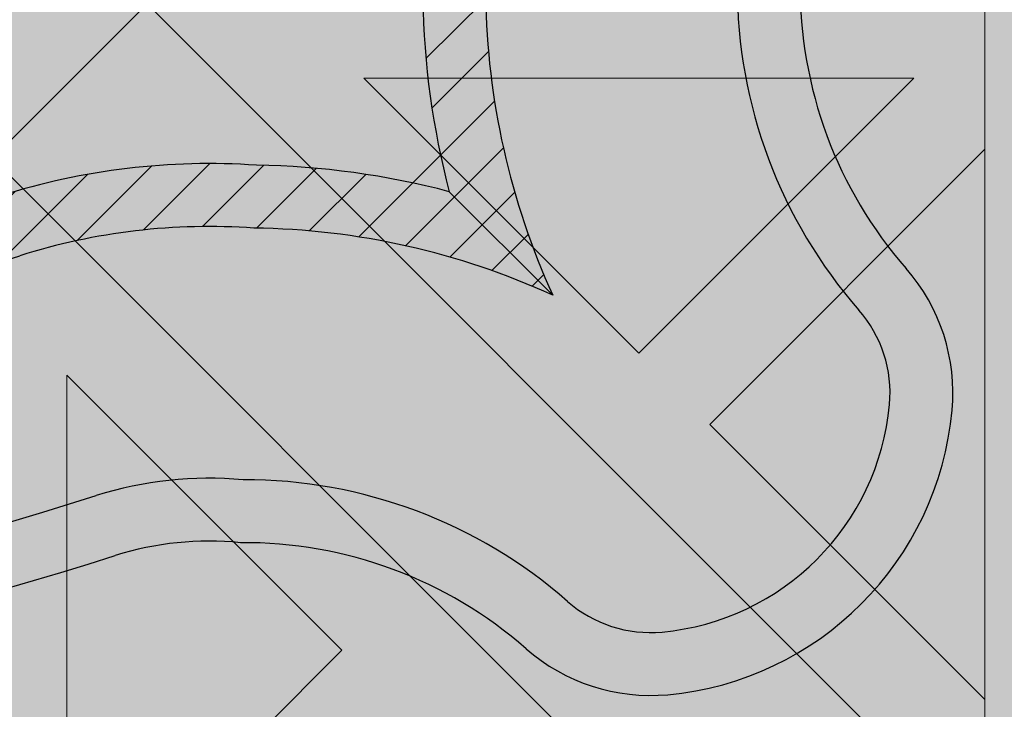
# Model space of a CAD drawing. Units: inches. Extents: x 844 to 2234, y 346 to 1084.
# Tile 54 of 93: x 1871.357 to 1873.853, y 692.527 to 694.275. Entities that reach past the tile are written whole.
import ezdxf

# ---------------------------------------------------------------- set-up
doc = ezdxf.new("R2010")
doc.units = ezdxf.units.IN
doc.header["$MEASUREMENT"] = 0
doc.layers.add('furniture', color=8, linetype='Continuous', lineweight=18)
doc.layers.add('RA-AP-01$0$INT', color=35, linetype='Continuous', lineweight=5)
doc.layers.add('RA-AP-01$0$FURN', color=3, linetype='Continuous')
doc.layers.add('RA-AP-01$0$WOOD', color=64, linetype='Continuous')

# ---------------------------------------------------------------- blocks, each defined once
blk = doc.blocks.new('A$C18D01794')
at = {"layer": 'RA-AP-01$0$INT'}
blk.add_hatch(color=256, dxfattribs=at).paths.add_polyline_path([(4.505206456958071, -6.306712009588038), (5.305206456958072, -6.306712009588038), (5.305206456958072, -7.106712009588038), (5.255206456951893, -7.10671200958804), (5.25520645694868, -6.356712009605972), (4.555206456959269, -6.356712009587461), (4.555206456956052, -7.106712009588038), (4.505206456958073, -7.106712009588038)])
h = blk.add_hatch(color=256, dxfattribs=at)
h.paths.add_polyline_path([(4.585917135068449, -6.356712009588271), (4.555206456959269, -6.35671200958746), (4.555206456959137, -6.387422687716308), (4.874495778835233, -6.706712009592356), (4.90520645695423, -6.676001331474049)])
h.paths.add_polyline_path([(5.255206456948813, -6.387422687716306), (5.255206456948682, -6.356712009605972), (5.224495778822613, -6.356712009605161), (4.905206456953498, -6.676001331474273), (4.935917135072151, -6.706712009592924)])
h.paths.add_polyline_path([(4.935917135072559, -6.706712009592068), (4.905206456953564, -6.737422687710376), (5.255206456951813, -7.087422687708613), (5.255206456951549, -7.026001331471008)])
h.paths.add_polyline_path([(4.555206456956399, -7.026001331471013), (4.555206456956134, -7.087422687708616), (4.905206456953821, -6.737422687710943), (4.874495778835166, -6.70671200959229)])
h = blk.add_hatch(color=256, dxfattribs=at)
h.paths.add_polyline_path([(4.585917135068448, -6.356712009588273), (4.614201406330596, -6.356712009589021), (4.668846067270487, -6.411356670531338), (4.723490728212344, -6.356712009591912), (4.771774999457151, -6.35671200959319), (4.826419660396886, -6.411356670535356), (4.862780050090322, -6.374996280843536), (4.844495778842715, -6.356712009595112), (4.862780050090411, -6.356712009595595), (4.905206456960182, -6.399138416468211), (4.947632863832445, -6.356712009597838), (4.965917135079675, -6.356712009598322), (4.947632863831759, -6.374996280845421), (4.983993253523576, -6.411356670538857), (5.038637914464627, -6.356712009600247), (5.08692218571208, -6.356712009601523), (5.141566846649976, -6.411356670541852), (5.196211507589851, -6.356712009604411), (5.224495778822615, -6.356712009605161), (4.905206456953975, -6.676001331473793)])
h.paths.add_polyline_path([(4.895206456956031, -6.637717060225675), (4.895206456958921, -6.528427738347902), (4.840561796018589, -6.583072399285802)], flags=16)
h.paths.add_polyline_path([(4.915206456955638, -6.637717060226121), (4.969851117895509, -6.583072399288678), (4.915206456957609, -6.528427738348344)], flags=16)
h.paths.add_polyline_path([(4.826419660395175, -6.568930263661755), (4.881064321335613, -6.514285602723745), (4.771774999456703, -6.514285602720857)], flags=16)
h.paths.add_polyline_path([(4.983993253519558, -6.568930263665262), (5.038637914460456, -6.514285602726792), (4.929348592581548, -6.514285602724816)], flags=16)
h.paths.add_polyline_path([(4.881064321336025, -6.494285602723742), (4.826419660397532, -6.439640941782821), (4.771774999457062, -6.494285602720859)], flags=16)
h.paths.add_polyline_path([(4.929348592582019, -6.494285602724817), (5.038637914460982, -6.494285602726792), (4.983993253522945, -6.439640941786327)], flags=16)
h.paths.add_polyline_path([(4.895206456960191, -6.480143467100443), (4.895206456962115, -6.407422687715913), (4.876922185715016, -6.389138416467584), (4.840561796021581, -6.425498806159401)], flags=16)
h.paths.add_polyline_path([(4.915206456958487, -6.480143467100889), (4.969851117899527, -6.425498806162279), (4.933490728206909, -6.389138416468043), (4.9152064569598, -6.40742268771434)], flags=16)
h.paths.add_polyline_path([(4.757632863832376, -6.480143467096812), (4.812277524772842, -6.425498806158772), (4.757632863834348, -6.370854145217844)], flags=16)
h.paths.add_polyline_path([(4.737632863832376, -6.480143467096286), (4.737632863834348, -6.370854145217375), (4.682988202893906, -6.425498806155385)], flags=16)
h.paths.add_polyline_path([(5.05278005008503, -6.480143467103376), (5.052780050087917, -6.370854145224413), (4.998135389146995, -6.425498806162908)], flags=16)
h.paths.add_polyline_path([(5.072780050085024, -6.480143467103744), (5.127424711025931, -6.42549880616527), (5.072780050087916, -6.370854145224832)], flags=16)
h.paths.add_polyline_path([(4.935917135072783, -6.706712009592292), (5.255206456948811, -6.387422687716309), (5.255206456948932, -6.415706958964177), (5.200561796010279, -6.470351619902839), (5.255206456949403, -6.524996280841948), (5.25520645694961, -6.5732805520894), (5.200561796009787, -6.627925213029239), (5.236922185702417, -6.664285602721864), (5.255206456949919, -6.646001331474357), (5.255206456949998, -6.664285602721898), (5.212780050078687, -6.706712009592262), (5.25520645695036, -6.749138416463932), (5.255206456950438, -6.767422687711313), (5.236922185702424, -6.749138416463297), (5.200561796009796, -6.785498806155928), (5.255206456950753, -6.840143467096874), (5.25520645695096, -6.888427738341682), (5.200561796010322, -6.943072399282328), (5.255206456951428, -6.997717060223427), (5.255206456951547, -7.026001331471006)])
h.paths.add_polyline_path([(5.042988202883395, -6.785498806155427), (5.097632863823085, -6.840143467095101), (5.097632863822622, -6.730854145216193)], flags=16)
h.paths.add_polyline_path([(5.028846067259663, -6.771356670531693), (5.083490728198774, -6.716712009592573), (4.974201406321001, -6.716712009593042)], flags=16)
h.paths.add_polyline_path([(5.117632863823087, -6.840143467095186), (5.172277524762331, -6.785498806155926), (5.11763286382262, -6.730854145216225)], flags=16)
h.paths.add_polyline_path([(5.08349072819877, -6.696712009593886), (5.028846067259652, -6.642067348654775), (4.974201406320998, -6.696712009593438)], flags=16)
h.paths.add_polyline_path([(5.131774999446817, -6.854285602718917), (5.186419660386065, -6.799640941779662), (5.241064321325782, -6.854285602719365)], flags=17)
h.paths.add_polyline_path([(5.131774999446228, -6.716712009592374), (5.186419660386065, -6.771356670532194), (5.222780050079488, -6.734996280838764), (5.204495778832781, -6.716712009592063)], flags=16)
h.paths.add_polyline_path([(5.097632863822613, -6.682569873970264), (5.097632863823061, -6.573280552091354), (5.042988202883383, -6.627925213031044)], flags=16)
h.paths.add_polyline_path([(5.131774999446899, -6.874285602718915), (5.241064321325809, -6.874285602719364), (5.186419660386591, -6.928930263658598)], flags=17)
h.paths.add_polyline_path([(5.131774999446226, -6.696712009594078), (5.204495778830767, -6.696712009594374), (5.22278005007868, -6.67842773834687), (5.186419660386049, -6.642067348654249)], flags=16)
h.paths.add_polyline_path([(5.11763286382262, -6.682569873970225), (5.17227752476232, -6.627925213030515), (5.117632863823064, -6.573280552091267)], flags=16)
h.paths.add_polyline_path([(5.186419660386069, -6.613783077405491), (5.241064321325754, -6.559138416465795), (5.131774999446791, -6.559138416466263)], flags=16)
h.paths.add_polyline_path([(5.131774999446872, -6.539138416466263), (5.24106432132578, -6.539138416465794), (5.186419660386554, -6.484493755526573)], flags=16)
h.paths.add_polyline_path([(5.255206456951811, -7.08742268770861), (5.255206456951895, -7.106712009588038), (4.555206456956052, -7.106712009588038), (4.555206456956136, -7.087422687708617), (4.905206456953973, -6.737422687710788)])
h.paths.add_polyline_path([(4.983993253513404, -6.8444937555241), (4.92934859257295, -6.899138416462108), (5.03863791445186, -6.899138416465014)], flags=16)
h.paths.add_polyline_path([(4.969851117889988, -6.83035161990006), (4.915206456952556, -6.775706958960171), (4.915206456949648, -6.884996280837944)], flags=16)
h.paths.add_polyline_path([(4.929348592572535, -6.919138416462105), (4.983993253511019, -6.973783077403037), (5.038637914451496, -6.919138416465012)], flags=16)
h.paths.add_polyline_path([(5.052780050074912, -6.93328055208906), (4.998135389134438, -6.987925213027088), (5.052780050072919, -7.042569873968025)], flags=16)
h.paths.add_polyline_path([(5.07278005007491, -6.933280552089588), (5.072780050072918, -7.042569873968497), (5.127424711013374, -6.987925213030498)], flags=16)
h.paths.add_polyline_path([(4.89520645695295, -6.775706958959721), (4.840561796013067, -6.830351619897157), (4.895206456950961, -6.884996280837494)], flags=16)
h.paths.add_polyline_path([(4.915206456948365, -6.933280552085403), (4.915206456946434, -7.006001331471951), (4.933490728192729, -7.024285602719066), (4.969851117886972, -6.987925213026453)], flags=16)
h.paths.add_polyline_path([(4.881064321327021, -6.899138416461022), (4.82641966038902, -6.84449375552057), (4.771774999448108, -6.899138416459029)], flags=16)
h.paths.add_polyline_path([(4.895206456950073, -6.933280552084951), (4.840561796009022, -6.987925213023558), (4.876922185700835, -7.024285602716997), (4.895206456948749, -7.006001331469487)], flags=16)
h.paths.add_polyline_path([(4.983993253510392, -7.0020673486505), (4.947632863816944, -7.038427738342319), (4.965917135064043, -7.05671200959023), (5.038637914448995, -7.056712009591555)], flags=16)
h.paths.add_polyline_path([(4.881064321326543, -6.91913841646102), (4.771774999447578, -6.919138416459031), (4.826419660385607, -6.973783077399508)], flags=16)
h.paths.add_polyline_path([(4.905206456946447, -7.014285602717636), (4.862780050074785, -7.056712009588352), (4.947632863816685, -7.056712009589775)], flags=16)
h.paths.add_polyline_path([(5.14156684663679, -7.002067348654549), (5.086922185696452, -7.056712009592438), (5.196211507574223, -7.056712009594425)], flags=16)
h.paths.add_polyline_path([(4.8264196603837, -7.002067348646972), (4.771774999442643, -7.056712009585575), (4.8444957788276, -7.056712009587508), (4.862780050075511, -7.038427738340416)], flags=16)
h.paths.add_polyline_path([(4.812277524760289, -6.98792521302292), (4.757632863822258, -6.933280552082447), (4.757632863819352, -7.042569873961408)], flags=16)
h.paths.add_polyline_path([(4.73763286382226, -6.933280552082079), (4.682988202881349, -6.987925213020536), (4.737632863819352, -7.04256987396099)], flags=16)
h.paths.add_polyline_path([(4.723490728195188, -7.056712009584289), (4.668846067257299, -7.002067348643949), (4.614201406317417, -7.056712009581383)], flags=16)
h.paths.add_polyline_path([(4.597632863829262, -6.706712009592262), (4.555206456957951, -6.664285602721896), (4.555206456958029, -6.646001331474357), (4.573490728205535, -6.664285602721864), (4.609851117898167, -6.627925213029238), (4.555206456958338, -6.573280552089402), (4.555206456958546, -6.524996280841952), (4.60985111789767, -6.470351619902839), (4.555206456959015, -6.415706958964177), (4.555206456959138, -6.387422687716309), (4.874495778835167, -6.70671200959229), (4.5552064569564, -7.026001331471015), (4.555206456956523, -6.997717060223433), (4.609851117897629, -6.94307239928233), (4.555206456956988, -6.888427738341681), (4.555206456957198, -6.840143467096881), (4.609851117898153, -6.78549880615593), (4.573490728205528, -6.749138416463297), (4.555206456957507, -6.76742268771132), (4.555206456957585, -6.749138416463933)])
h.paths.add_polyline_path([(4.712780050085332, -6.730854145216195), (4.712780050084863, -6.840143467095105), (4.767424711024555, -6.785498806155427)], flags=16)
h.paths.add_polyline_path([(4.726922185709173, -6.716712009592573), (4.781566846648288, -6.771356670531693), (4.836211507586949, -6.716712009593043)], flags=16)
h.paths.add_polyline_path([(4.692780050085327, -6.730854145216225), (4.638135389145619, -6.785498806155928), (4.692780050084865, -6.840143467095185)], flags=16)
h.paths.add_polyline_path([(4.726922185709182, -6.696712009593886), (4.836211507586949, -6.696712009593436), (4.7815668466483, -6.642067348654773)], flags=16)
h.paths.add_polyline_path([(4.678637914461726, -6.71671200959237), (4.605917135075169, -6.716712009592063), (4.587632863828464, -6.734996280838766), (4.623993253521887, -6.771356670532195)], flags=16)
h.paths.add_polyline_path([(4.712780050085336, -6.68256987397026), (4.767424711024568, -6.627925213031042), (4.71278005008489, -6.573280552091352)], flags=16)
h.paths.add_polyline_path([(4.678637914461726, -6.696712009594076), (4.623993253521899, -6.642067348654247), (4.587632863829271, -6.67842773834687), (4.605917135077185, -6.696712009594376)], flags=16)
h.paths.add_polyline_path([(4.692780050085336, -6.682569873970228), (4.692780050084889, -6.573280552091267), (4.638135389145632, -6.627925213030515)], flags=16)
h.paths.add_polyline_path([(4.623993253521885, -6.799640941779662), (4.678637914461131, -6.854285602718915), (4.56934859258217, -6.854285602719365)], flags=17)
h.paths.add_polyline_path([(4.623993253521901, -6.613783077405509), (4.678637914461158, -6.559138416466263), (4.569348592582195, -6.559138416465795)], flags=16)
h.paths.add_polyline_path([(4.678637914461051, -6.874285602718915), (4.623993253521361, -6.928930263658598), (4.569348592582143, -6.874285602719364)], flags=17)
h.paths.add_polyline_path([(4.678637914461076, -6.539138416466263), (4.623993253521399, -6.484493755526573), (4.569348592582167, -6.539138416465796)], flags=16)
h = blk.add_hatch(color=256, dxfattribs=at)
h.paths.add_polyline_path([(4.969851117891331, -6.583072399286455), (4.915206456952669, -6.63771706022511), (4.915206456952222, -6.528427738347337)])
h.paths.add_polyline_path([(4.895206456953064, -6.637717060225108), (4.840561796014413, -6.583072399286448), (4.895206456953533, -6.528427738347335)])
h.paths.add_polyline_path([(4.826419660390684, -6.568930263662714), (4.771774999451003, -6.514285602723024), (4.881064321329913, -6.514285602723489)])
h.paths.add_polyline_path([(4.881064321329884, -6.494285602723492), (4.771774999450921, -6.494285602723024), (4.82641966039018, -6.439640941783778)])
h.paths.add_polyline_path([(4.895206456953734, -6.48014346709988), (4.840561796013912, -6.425498806160046), (4.876922185707337, -6.389138416466622), (4.895206456954043, -6.40742268771333)])
h.paths.add_polyline_path([(4.862780050082808, -6.374996280843689), (4.826419660390178, -6.411356670536314), (4.771774999450351, -6.356712009596481), (4.844495778835303, -6.356712009596181)])
h.paths.add_polyline_path([(4.812277524766446, -6.425498806160041), (4.757632863827191, -6.480143467099289), (4.757632863826741, -6.370854145220329)])
h.paths.add_polyline_path([(4.737632863827191, -6.480143467099214), (4.682988202887508, -6.425498806159518), (4.737632863826743, -6.370854145220299)])
h.paths.add_polyline_path([(4.668846067263777, -6.41135667053579), (4.614201406325123, -6.356712009597128), (4.723490728202894, -6.356712009596675)])
h.paths.add_polyline_path([(4.905206456953846, -6.399138416467422), (4.862780050082654, -6.356712009596229), (4.947632863824561, -6.356712009595756)])
h.paths.add_polyline_path([(4.915206456952028, -6.480143467099882), (4.91520645695173, -6.407422687715346), (4.933490728199234, -6.389138416467428), (4.96985111789186, -6.425498806160055)])
h.paths.add_polyline_path([(5.038637914454841, -6.494285602723048), (4.929348592575874, -6.494285602723497), (4.983993253515593, -6.439640941783787)])
h.paths.add_polyline_path([(4.983993253515065, -6.568930263662725), (4.929348592575849, -6.514285602723495), (5.038637914454755, -6.514285602723045)])
h.paths.add_polyline_path([(5.052780050079843, -6.480143467099317), (4.998135389140595, -6.425498806160058), (5.052780050080309, -6.370854145220356)])
h.paths.add_polyline_path([(4.983993253516868, -6.411356670536324), (4.947632863824241, -6.374996280843694), (4.965917135071747, -6.356712009596188), (5.038637914456701, -6.356712009596504)])
h.paths.add_polyline_path([(5.127424711019533, -6.425498806159557), (5.072780050079843, -6.480143467099239), (5.07278005008031, -6.370854145220326)])
h.paths.add_polyline_path([(5.141566846643269, -6.411356670535829), (5.086922185704154, -6.356712009596707), (5.196211507581929, -6.356712009597176)])
h = blk.add_hatch(color=256, dxfattribs=at)
h.paths.add_polyline_path([(5.028846067259997, -6.642067348655121), (4.974201406321342, -6.696712009593783), (5.083490728199115, -6.69671200959423)])
h.paths.add_polyline_path([(4.974201406321344, -6.716712009593388), (5.028846067260004, -6.771356670532039), (5.083490728199117, -6.716712009592919)])
h.paths.add_polyline_path([(5.042988202883738, -6.785498806155768), (5.097632863823428, -6.840143467095449), (5.097632863822963, -6.73085414521654)])
h.paths.add_polyline_path([(5.117632863822961, -6.730854145216568), (5.117632863823428, -6.840143467095531), (5.172277524762674, -6.785498806156272)])
h.paths.add_polyline_path([(5.131774999446572, -6.716712009592718), (5.186419660386406, -6.77135667053254), (5.222780050079831, -6.734996280839116), (5.204495778833122, -6.716712009592409)])
h.paths.add_polyline_path([(5.236922185702764, -6.749138416463644), (5.200561796010139, -6.785498806156274), (5.255206456949971, -6.840143467096101), (5.255206456950271, -6.76742268771115)])
h.paths.add_polyline_path([(5.186419660386412, -6.799640941780006), (5.131774999447164, -6.854285602719262), (5.241064321326123, -6.854285602719711)])
h.paths.add_polyline_path([(5.131774999447238, -6.874285602719261), (5.186419660386934, -6.928930263658944), (5.241064321326153, -6.874285602719709)])
h.paths.add_polyline_path([(5.200561796010663, -6.943072399282675), (5.255206456949324, -6.997717060221329), (5.255206456949777, -6.888427738343558)])
h.paths.add_polyline_path([(5.21278005007903, -6.706712009592607), (5.255206456950223, -6.749138416463798), (5.255206456950696, -6.664285602721891)])
h.paths.add_polyline_path([(5.13177499944657, -6.696712009594424), (5.204495778831106, -6.696712009594723), (5.222780050079024, -6.678427738347219), (5.186419660386397, -6.642067348654592)])
h.paths.add_polyline_path([(5.117632863823405, -6.573280552091611), (5.117632863822955, -6.682569873970578), (5.172277524762665, -6.627925213030859)])
h.paths.add_polyline_path([(5.042988202883727, -6.627925213031387), (5.097632863822957, -6.682569873970603), (5.097632863823407, -6.573280552091697)])
h.paths.add_polyline_path([(5.131774999447135, -6.559138416466609), (5.186419660386394, -6.613783077405857), (5.241064321326097, -6.559138416466144)])
h.paths.add_polyline_path([(5.200561796010128, -6.627925213029584), (5.236922185702758, -6.664285602722211), (5.255206456950264, -6.646001331474705), (5.255206456949948, -6.573280552089752)])
h.paths.add_polyline_path([(5.186419660386895, -6.484493755526919), (5.131774999447213, -6.539138416466609), (5.241064321326127, -6.539138416466142)])
h.paths.add_polyline_path([(5.200561796010624, -6.470351619903183), (5.255206456949745, -6.524996280842298), (5.255206456949276, -6.415706958964523)])
for p, q in [((4.905206456953975, -6.676001331473793), (5.224495778822613, -6.356712009605161)), ((5.255206456951895, -7.106712009588038), (5.255206456948681, -6.356712009605972)), ((5.072780050085028, -6.48014346710374), (5.072780050087916, -6.37085414522483)), ((5.072780050087916, -6.37085414522483), (5.127424711025931, -6.42549880616527)), ((4.935917135072783, -6.706712009592292), (5.255206456948813, -6.387422687716307)), ((5.255206456948934, -6.415706958964177), (5.200561796010281, -6.470351619902839)), ((5.12742471102593, -6.425498806165272), (5.072780050085028, -6.48014346710374)), ((5.255206456949399, -6.524996280841946), (5.200561796010281, -6.470351619902839)), ((5.18641966038655, -6.484493755526575), (5.131774999446872, -6.539138416466263)), ((5.241064321325782, -6.539138416465796), (5.186419660386552, -6.484493755526573)), ((5.131774999446872, -6.539138416466263), (5.241064321325782, -6.539138416465796))]:
    blk.add_line(p, q, dxfattribs=at)
blk = doc.blocks.new('A$C32926AE1')
at = {"layer": 'RA-AP-01$0$WOOD'}
h = blk.add_hatch(color=256, dxfattribs=at)
h.dxf.hatch_style = 1
h.paths.add_polyline_path([(5.157430609644524, 4.573483066760929, -0.1009492694046607), (5.155401577623758, 4.593365984175333, -0.1842662638101597), (5.172249623284174, 4.638795604568598, 0.2056608120311276), (5.179560981299304, 4.661316324430096, 0.3614336704623542), (5.134352340494423, 4.706524965234944, 0.2056608120311297), (5.111831620632933, 4.699213607219793, -0.1842662638101113), (5.066402000239693, 4.682365561559342, -0.1055311479399994), (5.045656153913092, 4.68467289944697, 0.1567636581983829), (4.763886414745334, 4.684672899446966, -0.1055311479399895), (4.743140568418733, 4.68236556155934, -0.1842662638100833), (4.6977109480255, 4.69921360721979, 0.2056608120302612), (4.675190228164109, 4.706524965234949, 0.3614336704708441), (4.629981587358889, 4.66131632442871, 0.2056608120245944), (4.637292945374126, 4.638795604567974, -0.1842662638101024), (4.654140991034615, 4.59336598417475, -0.1009492694055169), (4.652111959013835, 4.573483066760181, 0.021410119221476), (4.629748025606143, 4.156712009541676, 0.0214101192214795), (4.652111959013809, 3.739940952323101, -0.1009492694059586), (4.654140991034615, 3.720058034908448, -0.1842662638100975), (4.637292945374126, 3.674628414515226, 0.2056608120245705), (4.629981587358889, 3.652107694654492, 0.3614336704708879), (4.675190228164113, 3.606899053848249, 0.2056608120302384), (4.697710948025501, 3.614210411863408, -0.1842662638100995), (4.743140568418738, 3.63105845752386, -0.1055311479402541), (4.763886414745388, 3.628751119636215, 0.1567636581983776), (5.045656153913137, 3.628751119636244, -0.1055311479397538), (5.066402000239692, 3.631058457523857, -0.1842662638101067), (5.111831620632931, 3.614210411863407, 0.2056608120310924), (5.134352340494417, 3.606899053848256, 0.3614336704624001), (5.179560981299307, 3.652107694653103, 0.2056608120311314), (5.172249623284175, 3.6746284145146, -0.1842662638101402), (5.155401577623758, 3.72005803490786, -0.1009492694051366), (5.15743060964455, 3.739940952322354, 0.0214101192215073), (5.179794543052287, 4.156712009541468, 0.0214101192215252)])
h.paths.add_polyline_path([(4.639748609479751, 4.156712009541513, 0.0213537860821624), (4.661970494867118, 3.741887061152232, -0.094075836301374), (4.664143710413708, 3.7196126951003, -0.1824818158568985), (4.644813765429836, 3.668037719127816, 0.2056608120245319), (4.639939526753007, 3.653023905887301, 0.3614336704710246), (4.676106439397173, 3.616856993242342, 0.2056608120302234), (4.691120252638095, 3.621731231919122, -0.1824818158602558), (4.742695228611606, 3.641061176902986, -0.1029891339458722), (4.766991894714349, 3.638256818950944, 0.156709409989566), (5.042550673941472, 3.638256818950105, -0.102989133958497), (5.066847340047078, 3.641061176902949, -0.1824818158594995), (5.118422316020358, 3.621731231919103, 0.2056608120311416), (5.133436129261316, 3.616856993242346, 0.3614336704621468), (5.169603041905217, 3.653023905886178, 0.2056608120310986), (5.164728803228477, 3.668037719127177, -0.1824818158565612), (5.145398858244737, 3.719612695099578, -0.0940758363009313), (5.147572073791232, 3.741887061151398, 0.0213537860822023), (5.169793959178681, 4.156712009541451, 0.0213537860822226), (5.147572073791203, 4.571536957931898, -0.0940758363005034), (5.145398858244737, 4.59381132398362, -0.1824818158565587), (5.164728803228476, 4.645386299956021, 0.2056608120311045), (5.169603041905216, 4.66040011319702, 0.3614336704621845), (5.133436129261313, 4.696567025840856, 0.2056608120310773), (5.118422316020359, 4.691692787164098, -0.182481815859508), (5.066847340047078, 4.67236284218025, -0.1029891339584606), (5.04255067394148, 4.675167200133092, 0.156709409989566), (4.766991894714357, 4.675167200132257, -0.1029891339458842), (4.742695228611611, 4.672362842180213, -0.1824818158602725), (4.691120252638095, 4.691692787164077, 0.2056608120302152), (4.676106439397174, 4.696567025840858, 0.3614336704710363), (4.639939526753005, 4.660400113195899, 0.2056608120245495), (4.644813765429837, 4.645386299955384, -0.1824818158568934), (4.664143710413708, 4.593811323982902, -0.0940758363009187), (4.661970494867149, 4.571536957931074, 0.021353786082177)], flags=16)
h.paths.add_polyline_path([(5.129794543052235, 4.432167055276933, -0.0141661062790638), (5.130152669293814, 4.156927903047693, -0.0141661062790647), (5.129794543052234, 3.881688750818433, -0.0785247771143638), (5.10979738006795, 3.755143611847103, 0.0945969212073497), (5.105408519571111, 3.717898134952927, 0.1043170707844957), (5.116074640131521, 3.670385395016088, 0.1043170707864965), (5.068561900193738, 3.681051515576561, 0.09459692119553), (5.031316423304057, 3.676662655080835, -0.1580239521427272), (4.778226145355827, 3.676662655080367, 0.0945969211986668), (4.740980668464973, 3.681051515576592, 0.1043170707882822), (4.693467928526415, 3.670385395015844, 0.1043170707867916), (4.704134049087309, 3.717898134953662, 0.0945969211972894), (4.69974518859162, 3.755143611844042, -0.0785247771163196), (4.679748025606343, 3.881688750818406, -0.0141661062790663), (4.679389899364763, 4.156927903047693, -0.0141661062790672), (4.679748025606343, 4.432167055276998, -0.0785247771163064), (4.699745188591625, 4.55871219425134, 0.094596921197333), (4.704134049087308, 4.595957671141738, 0.1043170707867205), (4.693467928526416, 4.643470411079523, 0.1043170707882628), (4.740980668464965, 4.632804290518776, 0.0945969211988114), (4.778226145355874, 4.637193151015016, -0.158023952142669), (5.031316423304015, 4.637193151014546, 0.0945969211956361), (5.068561900193736, 4.632804290518806, 0.1043170707864979), (5.11607464013152, 4.643470411079278, 0.1043170707844617), (5.105408519571112, 4.595957671142455, 0.0945969212074597), (5.109797380067959, 4.558712194248236, -0.0785247771143467)], flags=0)
h.paths.add_polyline_path([(5.119794532311105, 4.432259799204851, -0.0142000800617244), (5.120156169157484, 4.156927903047701, -0.0142000800617277), (5.119794532311105, 3.881596006890482, -0.0784894509520253), (5.100273383573699, 3.758192358677797, 0.0940138827242913), (5.095413455884425, 3.717477693979438, 0.0606271852308753), (5.099615656341024, 3.686844378806616, 0.0606271852322524), (5.068982341167493, 3.691046579263239, 0.0940138827010453), (5.028267676478798, 3.686186651576848, -0.1580706864508061), (4.781274892180912, 3.686186651576435, 0.0940138827026903), (4.740560227491556, 3.691046579263279, 0.0606271852339895), (4.709926912317155, 3.686844378806508, 0.0606271852329405), (4.714129112773991, 3.717477693980356, 0.094013882701304), (4.709269185087677, 3.758192358669163, -0.0784894509577193), (4.689748036347473, 3.881596006890469, -0.014200080061729), (4.689386399501094, 4.156927903047709, -0.0142000800617217), (4.689748036347473, 4.432259799204808, -0.078489450957724), (4.709269185087651, 4.555663447426125, 0.0940138827014585), (4.714129112773992, 4.596378112114996, 0.0606271852329731), (4.709926912317154, 4.62701142728886, 0.0606271852340196), (4.74056022749157, 4.622809226832087, 0.0940138827024997), (4.781274892180847, 4.627669154518912, -0.1580706864508359), (5.028267676478777, 4.627669154518526, 0.0940138827010946), (5.068982341167492, 4.622809226832129, 0.060627185232254), (5.099615656341024, 4.627011427288751, 0.0606271852308727), (5.095413455884425, 4.59637811211593, 0.0940138827241088), (5.100273383573675, 4.555663447417647, -0.0784894509520978)], flags=0)
h.paths.add_polyline_path([(5.06978912287499, 4.430218106756144, -0.014241683694547), (5.070173729147532, 4.156927903047672, -0.0142416836945458), (5.06978912287499, 3.883637699339223, -0.0800609523125196), (5.052662118612511, 3.773463122773442, 0.0526421978001116), (5.04590916754064, 3.740550867606997, 0.0526421977992423), (5.012996912374707, 3.73379791653534, -0.1583028414718258), (4.796545656286308, 3.73379791653451, 0.0526421978034211), (4.763633401117837, 3.740550867607021, 0.0526421978018622), (4.756880450045755, 3.773463122774558, -0.0800609523117106), (4.739753445783639, 3.883637699339268, -0.0142416836945435), (4.739368839511098, 4.156927903047671, -0.0142416836945477), (4.739753445783639, 4.430218106756155, -0.0800609523116345), (4.75688045004574, 4.540392683320762, 0.052642197801941), (4.763633401117837, 4.573304938488346, 0.0526421978035071), (4.796545656286361, 4.580057889560873, -0.1583028414717561), (5.012996912374669, 4.580057889560039, 0.0526421977993048), (5.04590916754064, 4.57330493848837, 0.0526421978002057), (5.052662118612529, 4.540392683321868, -0.080060952312477)], flags=0)
h.paths.add_polyline_path([(5.049789715110557, 4.43038092723357, -0.0143097550741839), (5.05018085590259, 4.156927903047715, -0.0143097550741854), (5.049789715110558, 3.883474878861827, -0.0800685599149176), (5.03362098255317, 3.779581877367999, 0.0306258898956367), (5.028241146483733, 3.758218888663947, 0.0306258898977031), (5.006878157778253, 3.75283905259408, -0.1583983521624096), (4.802664410878162, 3.752839052594731, 0.0306258898946014), (4.781301422174808, 3.758218888663924, 0.0306258898967912), (4.775921586105202, 3.779581877368794, -0.080068559914251), (4.759752853548071, 3.883474878861786, -0.0143097550741854), (4.759361712756037, 4.156927903047671, -0.0143097550741854), (4.759752853548071, 4.430380927233557, -0.0800685599142479), (4.775921586105193, 4.534273928726546, 0.0306258898968306), (4.781301422174808, 4.555636917431444, 0.0306258898945754), (4.802664410878143, 4.561016753500631, -0.1583983521624168), (5.006878157778244, 4.561016753501291, 0.0306258898977177), (5.028241146483733, 4.555636917431421, 0.0306258898958182), (5.03362098255321, 4.534273928727244, -0.080068559914796)], flags=0)
h.paths.add_polyline_path([(4.999766070382627, 4.428171244713864, -0.0143443147609634), (5.000198441819402, 4.156927903047689, -0.0143443147609612), (4.999766070382627, 3.885684561381556, -0.0784641635803329), (4.987356730658798, 3.799103304488872, -0.1506053783831347), (4.822185837999821, 3.79910330448882, -0.0784641635803318), (4.809776498276007, 3.885684561381509, -0.014344314760963), (4.809344126839227, 4.156927903047677, -0.0143443147609645), (4.809776498276007, 4.428171244713873, -0.0784641635803192), (4.822185837999822, 4.514752501606549, -0.1506053783831338), (4.987356730658798, 4.514752501606494, -0.078464163580285)], flags=0)
h.paths.add_polyline_path([(4.979755254238824, 4.42764379880488, -0.0143772539198268), (4.980205517789977, 4.156927903047693, -0.0143772539198275), (4.979755254238824, 3.886212007290489, -0.0689242507424422), (4.971183264704897, 3.815276770442801, -0.1296645318904179), (4.838359303953726, 3.815276770442746, -0.0689242507424186), (4.829787314419809, 3.886212007290419, -0.0143772539198292), (4.829337050868653, 4.156927903047653, -0.0143772539198325), (4.829787314419809, 4.427643798804946, -0.0689242507424211), (4.838359303953725, 4.498579035652621, -0.1296645318904187), (4.971183264704897, 4.498579035652565, -0.0689242507424401)], flags=0)
h = blk.add_hatch(color=256, dxfattribs=at)
h.dxf.hatch_style = 1
h.paths.add_polyline_path([(5.145398858244737, 4.59381132398362, -0.1824818158565616), (5.164728803228476, 4.645386299956021, 0.2056608120311045), (5.169603041905216, 4.66040011319702, 0.3614336704621845), (5.133436129261313, 4.696567025840856, 0.2056608120310773), (5.118422316020359, 4.691692787164098, -0.182481815859508), (5.066847340047078, 4.67236284218025, -0.1029891339584606), (5.04255067394148, 4.675167200133092, 0.156709409989566), (4.766991894714357, 4.675167200132257, -0.1029891339458842), (4.742695228611611, 4.672362842180213, -0.1824818158602725), (4.691120252638095, 4.691692787164077, 0.2056608120302152), (4.676106439397174, 4.696567025840858, 0.3614336704710363), (4.639939526753005, 4.660400113195899, 0.2056608120245495), (4.644813765429837, 4.645386299955384, -0.1824818158568934), (4.664143710413708, 4.593811323982902, -0.0940758363009187), (4.661970494867149, 4.571536957931074, 0.0213537860821772), (4.639748609479751, 4.156712009541507, 0.0213537860821625), (4.661970494867119, 3.741887061152226, -0.0940758363013071), (4.664143710413708, 3.719612695100309, -0.1824818158569294), (4.644813765429836, 3.668037719127816, 0.2056608120245319), (4.639939526753007, 3.653023905887301, 0.3614336704710246), (4.676106439397173, 3.616856993242342, 0.2056608120302234), (4.691120252638095, 3.621731231919122, -0.1824818158602558), (4.742695228611606, 3.641061176902986, -0.1029891339458722), (4.766991894714349, 3.638256818950944, 0.156709409989566), (5.042550673941472, 3.638256818950105, -0.102989133958497), (5.066847340047078, 3.641061176902949, -0.1824818158594995), (5.118422316020358, 3.621731231919103, 0.2056608120311416), (5.133436129261316, 3.616856993242346, 0.3614336704621468), (5.169603041905217, 3.653023905886178, 0.2056608120310986), (5.164728803228477, 3.668037719127177, -0.1824818158565612), (5.145398858244737, 3.719612695099578, -0.0940758363009313), (5.147572073791232, 3.741887061151398, 0.0213537860822023), (5.169793959178681, 4.156712009541451, 0.0213537860822226), (5.147572073791203, 4.571536957931898, -0.0940758363004996)])
h.paths.add_polyline_path([(5.109797380067958, 4.55871219424824, -0.0785247771143472), (5.129794543052234, 4.432167055276936, -0.0141661062790644), (5.130152669293814, 4.156927903047685, -0.014166106279066), (5.129794543052234, 3.881688750818401, -0.0785247771143517), (5.109797380067946, 3.755143611847092, 0.0945969212073132), (5.105408519571111, 3.717898134952929, 0.1043170707844995), (5.116074640131521, 3.670385395016088, 0.1043170707864965), (5.068561900193738, 3.681051515576561, 0.09459692119553), (5.031316423304057, 3.676662655080835, -0.1580239521427272), (4.778226145355827, 3.676662655080367, 0.0945969211986668), (4.740980668464973, 3.681051515576592, 0.1043170707882822), (4.693467928526415, 3.670385395015844, 0.1043170707867916), (4.704134049087309, 3.717898134953662, 0.0945969211972894), (4.69974518859162, 3.755143611844042, -0.0785247771163196), (4.679748025606343, 3.881688750818406, -0.0141661062790663), (4.679389899364763, 4.156927903047693, -0.0141661062790672), (4.679748025606343, 4.432167055276998, -0.0785247771163064), (4.699745188591625, 4.55871219425134, 0.094596921197333), (4.704134049087308, 4.595957671141738, 0.1043170707867205), (4.693467928526416, 4.643470411079523, 0.1043170707882628), (4.740980668464965, 4.632804290518776, 0.0945969211988114), (4.778226145355874, 4.637193151015016, -0.158023952142669), (5.031316423304015, 4.637193151014546, 0.0945969211956361), (5.068561900193736, 4.632804290518806, 0.1043170707864979), (5.11607464013152, 4.643470411079278, 0.1043170707844617), (5.105408519571112, 4.595957671142455, 0.0945969212074504)], flags=16)
h.paths.add_polyline_path([(5.100273383573655, 4.55566344741771, -0.0784894509521388), (5.119794532311105, 4.432259799204852, -0.0142000800617252), (5.120156169157484, 4.156927903047686, -0.014200080061726), (5.119794532311105, 3.881596006890502, -0.0784894509520446), (5.100273383573696, 3.758192358677786, 0.0940138827242721), (5.095413455884425, 3.717477693979436, 0.0606271852308692), (5.099615656341024, 3.686844378806616, 0.0606271852322522), (5.068982341167493, 3.691046579263239, 0.0940138827010453), (5.028267676478798, 3.686186651576848, -0.1580706864508061), (4.781274892180912, 3.686186651576435, 0.0940138827026903), (4.740560227491556, 3.691046579263279, 0.0606271852339895), (4.709926912317155, 3.686844378806508, 0.0606271852329405), (4.714129112773991, 3.717477693980356, 0.094013882701304), (4.709269185087677, 3.758192358669163, -0.0784894509577193), (4.689748036347473, 3.881596006890469, -0.014200080061729), (4.689386399501094, 4.156927903047709, -0.0142000800617217), (4.689748036347473, 4.432259799204808, -0.078489450957724), (4.709269185087651, 4.555663447426125, 0.0940138827014585), (4.714129112773992, 4.596378112114996, 0.0606271852329731), (4.709926912317154, 4.62701142728886, 0.0606271852340196), (4.74056022749157, 4.622809226832087, 0.0940138827024997), (4.781274892180847, 4.627669154518912, -0.1580706864508359), (5.028267676478777, 4.627669154518526, 0.0940138827010946), (5.068982341167492, 4.622809226832129, 0.060627185232254), (5.099615656341024, 4.627011427288751, 0.0606271852308727), (5.095413455884425, 4.59637811211593, 0.094013882723957)], flags=0)
h.paths.add_polyline_path([(5.04590916754064, 4.57330493848837, 0.0526421978002057), (5.052662118612529, 4.540392683321868, -0.0800609523124783), (5.06978912287499, 4.430218106756142, -0.0142416836945469), (5.070173729147532, 4.156927903047672, -0.0142416836945458), (5.06978912287499, 3.883637699339223, -0.0800609523125196), (5.052662118612511, 3.773463122773442, 0.0526421978001116), (5.04590916754064, 3.740550867606997, 0.0526421977992423), (5.012996912374707, 3.73379791653534, -0.1583028414718258), (4.796545656286308, 3.73379791653451, 0.0526421978034211), (4.763633401117837, 3.740550867607021, 0.0526421978018622), (4.756880450045755, 3.773463122774558, -0.0800609523117106), (4.739753445783639, 3.883637699339268, -0.0142416836945435), (4.739368839511098, 4.156927903047671, -0.0142416836945477), (4.739753445783639, 4.430218106756155, -0.0800609523116345), (4.75688045004574, 4.540392683320762, 0.052642197801941), (4.763633401117837, 4.573304938488346, 0.0526421978035071), (4.796545656286361, 4.580057889560873, -0.1583028414717561), (5.012996912374669, 4.580057889560039, 0.0526421977993048)], flags=0)
h.paths.add_polyline_path([(5.028241146483733, 4.555636917431422, 0.0306258898956949), (5.033620982553182, 4.534273928727329, -0.0800685599148649), (5.049789715110557, 4.430380927233569, -0.0143097550741839), (5.05018085590259, 4.156927903047715, -0.0143097550741854), (5.049789715110558, 3.883474878861827, -0.0800685599149176), (5.03362098255317, 3.779581877367999, 0.0306258898956367), (5.028241146483733, 3.758218888663947, 0.0306258898977031), (5.006878157778253, 3.75283905259408, -0.1583983521624096), (4.802664410878162, 3.752839052594731, 0.0306258898946014), (4.781301422174808, 3.758218888663924, 0.0306258898967912), (4.775921586105202, 3.779581877368794, -0.080068559914251), (4.759752853548071, 3.883474878861786, -0.0143097550741854), (4.759361712756037, 4.156927903047671, -0.0143097550741854), (4.759752853548071, 4.430380927233557, -0.0800685599142479), (4.775921586105193, 4.534273928726546, 0.0306258898968306), (4.781301422174808, 4.555636917431444, 0.0306258898945754), (4.802664410878143, 4.561016753500631, -0.1583983521624168), (5.006878157778244, 4.561016753501291, 0.0306258898977174)], flags=0)
h.paths.add_polyline_path([(4.987356730658798, 4.514752501606494, -0.0784641635803018), (4.999766070382627, 4.428171244713845, -0.0143443147609637), (5.000198441819402, 4.156927903047665, -0.0143443147609622), (4.999766070382628, 3.885684561381514, -0.0784641635802952), (4.987356730658797, 3.799103304488872, -0.1506053783831338), (4.822185837999821, 3.799103304488819, -0.0784641635803342), (4.809776498276007, 3.885684561381512, -0.0143443147609628), (4.809344126839227, 4.156927903047676, -0.0143443147609646), (4.809776498276007, 4.428171244713873, -0.0784641635803192), (4.822185837999822, 4.514752501606549, -0.1506053783831338)], flags=0)
h.paths.add_polyline_path([(4.971183264704897, 4.498579035652566, -0.0689242507424384), (4.979755254238824, 4.427643798804883, -0.0143772539198276), (4.980205517789977, 4.15692790304768, -0.0143772539198258), (4.979755254238823, 3.88621200729051, -0.0689242507424628), (4.971183264704897, 3.815276770442801, -0.129664531890417), (4.838359303953726, 3.815276770442746, -0.0689242507424186), (4.829787314419809, 3.886212007290419, -0.0143772539198292), (4.829337050868653, 4.156927903047653, -0.0143772539198325), (4.829787314419809, 4.427643798804946, -0.0689242507424211), (4.838359303953725, 4.498579035652621, -0.1296645318904187)], flags=0)
h = blk.add_hatch(dxfattribs=at)
h.set_pattern_fill('ANSI31', color=256, scale=0.05, style=0)
h.set_pattern_definition([(45, (0, 0), (-0.0044194173824159, 0.0044194173824159), [])])
h.paths.add_polyline_path([(5.130152669293814, 4.156927903047704, 0.0141661062790657), (5.129794543052234, 4.432167055276982, 0.0777827904001433), (5.110168979996553, 4.557559993161921, -0.0976515123401879), (5.105408519571111, 4.595957671142454, -0.1043170707844687), (5.116074640131522, 4.64347041107928), (5.099615656341024, 4.627011427288751, 0.0606271852308727), (5.095413455884425, 4.59637811211593, 0.0940138827241088), (5.100273383573675, 4.555663447417647, -0.0784894509520972), (5.119794532311105, 4.432259799204852, -0.0142000800617252), (5.120156169157484, 4.156927903047686, -0.014200080061726), (5.119794532311105, 3.881596006890502, -0.0784894509520446), (5.100273383573696, 3.758192358677786, 0.0940138827242721), (5.095413455884425, 3.717477693979436, 0.0606271852308692), (5.099615656341024, 3.686844378806616), (5.116074640131519, 3.67038539501609, -0.1043170707844594), (5.105408519571112, 3.717898134952912, -0.0976515123401594), (5.11016897999655, 3.756295812933435, 0.0777827904001654), (5.129794543052234, 3.881688750818409, 0.0141661062790665)])
h.paths.add_polyline_path([(5.030164222210597, 3.676291055149937, -0.0976515123472002), (5.068561900193739, 3.681051515576561, -0.1043170707864927), (5.116074640131521, 3.670385395016088), (5.099615656341024, 3.686844378806616, 0.0606271852322522), (5.068982341167493, 3.691046579263239, 0.0940138827010453), (5.028267676478798, 3.686186651576848, -0.1580706864508061), (4.781274892180912, 3.686186651576435, 0.0940138827026903), (4.740560227491556, 3.691046579263279, 0.0606271852339913), (4.709926912317154, 3.686844378806508), (4.693467928526416, 3.670385395015845, -0.1043170707882796), (4.740980668464973, 3.681051515576592, -0.0976515123427246), (4.779378346446416, 3.676291055150394, 0.156512506893803)])
h.paths.add_polyline_path([(4.689748036347473, 3.881596006890472, -0.014200080061729), (4.689386399501094, 4.156927903047712, -0.0142000800617195), (4.689748036347473, 4.432259799204768, -0.078489450957742), (4.709269185087648, 4.555663447426114, 0.0940138827014821), (4.714129112773992, 4.596378112114995, 0.0606271852329748), (4.709926912317154, 4.62701142728886), (4.693467928526414, 4.643470411079524, -0.1043170707867939), (4.704134049087309, 4.595957671141706, -0.09765151234893), (4.699373588660725, 4.557559993157876, 0.0777827903975372), (4.679748025606343, 4.432167055276987, 0.0141661062790675), (4.679389899364763, 4.156927903047675, 0.0141661062790641), (4.679748025606343, 3.88168875081843, 0.0777827903975637), (4.699373588660724, 3.756295812937497, -0.0976515123490278), (4.704134049087308, 3.717898134953629, -0.1043170707867196), (4.693467928526416, 3.670385395015845), (4.709926912317155, 3.686844378806508, 0.0606271852329413), (4.714129112773991, 3.717477693980357, 0.0940138827013084), (4.709269185087676, 3.758192358669166, -0.0784894509577192)])
h.paths.add_polyline_path([(4.779378346446434, 4.63756475094498, -0.0976515123427943), (4.740980668464964, 4.632804290518776, -0.1043170707882609), (4.693467928526416, 4.643470411079523), (4.709926912317154, 4.62701142728886, 0.0606271852340196), (4.74056022749157, 4.622809226832087, 0.0940138827024997), (4.781274892180847, 4.627669154518912, -0.1580706864508359), (5.028267676478777, 4.627669154518526, 0.0940138827010946), (5.068982341167492, 4.622809226832129, 0.060627185232254), (5.099615656341024, 4.627011427288751), (5.116074640131521, 4.643470411079279, -0.1043170707865022), (5.068561900193735, 4.632804290518806, -0.0976515123475899), (5.030164222210446, 4.637564750945479, 0.1565125068936924)])
h = blk.add_hatch(dxfattribs=at)
h.set_pattern_fill('ANSI32', color=256, scale=0.2, style=0)
h.set_pattern_definition([(45, (0, 0), (-0.0530330085889911, 0.0530330085889911), []), (45, (0.035355339, 0), (-0.0530330085889911, 0.0530330085889911), [])])
h.paths.add_polyline_path([(5.119794532311105, 4.432259799204823, 0.0777015974868765), (5.10065834347252, 4.554469821747928, -0.0968902511992216), (5.095413455884425, 4.596378112115931, -0.060627185230871), (5.099615656341024, 4.627011427288751, -0.060627185232254), (5.068982341167492, 4.622809226832129, -0.0968902512198245), (5.027074050790956, 4.628054114423209, 0.1564657949319105), (4.782468517866163, 4.628054114422785, -0.0968902512152247), (4.740560227491555, 4.622809226832088, -0.0606271852339878), (4.709926912317155, 4.627011427288859, -0.0606271852329413), (4.714129112773991, 4.596378112115011, -0.0968902512205338), (4.708884225182929, 4.554469821738175, 0.0777015974804443), (4.689748036347473, 4.43225979920482, 0.0142000800617215), (4.689386399501094, 4.156927903047726, 0.0142000800617273), (4.689748036347473, 3.88159600689052, 0.077701597480541), (4.708884225182985, 3.759385984357019, -0.096890251220082), (4.714129112773992, 3.717477693980371, -0.0606271852329731), (4.709926912317154, 3.686844378806507, -0.060627185233988), (4.740560227491554, 3.691046579263279, -0.0968902512152569), (4.782468517866175, 3.685801691672578, 0.1564657949319236), (5.027074050790988, 3.685801691672169, -0.0968902512197451), (5.068982341167491, 3.691046579263239, -0.0606271852322557), (5.099615656341024, 3.686844378806616, -0.0606271852308727), (5.095413455884425, 3.717477693979438, -0.0968902511991229), (5.100658343472507, 3.7593859843474, 0.0777015974868745), (5.119794532311105, 3.8815960068905, 0.014200080061726), (5.120156169157484, 4.156927903047685, 0.0142000800617238)])
h.paths.add_polyline_path([(5.070173729147531, 4.156927903047684, -0.0142416836945481), (5.06978912287499, 3.883637699339191, -0.0800609523125107), (5.052662118612505, 3.773463122773424, 0.0526421978000811), (5.04590916754064, 3.740550867606997, 0.0526421977993214), (5.012996912374658, 3.733797916535325, -0.1583028414717916), (4.796545656286304, 3.733797916534512, 0.0526421978034138), (4.763633401117837, 3.740550867607021, 0.0526421978018622), (4.756880450045755, 3.773463122774558, -0.0800609523117106), (4.739753445783639, 3.883637699339268, -0.0142416836945435), (4.739368839511098, 4.156927903047671, -0.0142416836945477), (4.739753445783639, 4.430218106756155, -0.0800609523116345), (4.75688045004574, 4.540392683320762, 0.052642197801941), (4.763633401117837, 4.573304938488346, 0.0526421978035071), (4.796545656286361, 4.580057889560873, -0.1583028414717561), (5.012996912374669, 4.580057889560039, 0.0526421977993048), (5.04590916754064, 4.57330493848837, 0.0526421978002057), (5.052662118612529, 4.540392683321868, -0.0800609523124783), (5.06978912287499, 4.430218106756142, -0.0142416836945463)], flags=16)
h.paths.add_polyline_path([(5.050180855902591, 4.156927903047686, -0.0143097550741856), (5.049789715110558, 3.883474878861795, -0.0800685599148126), (5.033620982553202, 3.7795818773681, 0.0306258898957837), (5.028241146483733, 3.758218888663947, 0.0306258898977031), (5.006878157778253, 3.75283905259408, -0.1583983521624096), (4.802664410878162, 3.752839052594731, 0.0306258898946014), (4.781301422174808, 3.758218888663924, 0.0306258898967912), (4.775921586105202, 3.779581877368794, -0.080068559914251), (4.759752853548071, 3.883474878861786, -0.0143097550741854), (4.759361712756037, 4.156927903047671, -0.0143097550741854), (4.759752853548071, 4.430380927233557, -0.0800685599142479), (4.775921586105193, 4.534273928726546, 0.0306258898968306), (4.781301422174808, 4.555636917431444, 0.0306258898945754), (4.802664410878143, 4.561016753500631, -0.1583983521624168), (5.006878157778244, 4.561016753501291, 0.0306258898977177), (5.028241146483733, 4.555636917431421, 0.0306258898958182), (5.03362098255321, 4.534273928727244, -0.0800685599147973), (5.049789715110557, 4.430380927233568, -0.0143097550741854)], flags=0)
h.paths.add_polyline_path([(5.000198441819402, 4.15692790304769, -0.0143443147609622), (4.999766070382627, 3.885684561381539, -0.0784641635803169), (4.987356730658798, 3.799103304488873, -0.1506053783831347), (4.822185837999821, 3.79910330448882, -0.0784641635803318), (4.809776498276007, 3.885684561381509, -0.014344314760963), (4.809344126839227, 4.156927903047677, -0.0143443147609645), (4.809776498276007, 4.428171244713873, -0.0784641635803192), (4.822185837999822, 4.514752501606549, -0.1506053783831338), (4.987356730658798, 4.514752501606494, -0.0784641635803018), (4.999766070382627, 4.428171244713845, -0.0143443147609624)], flags=0)
h.paths.add_polyline_path([(4.980205517789976, 4.156927903047707, -0.0143772539198295), (4.979755254238824, 3.886212007290466, -0.06892425074242), (4.971183264704897, 3.815276770442801, -0.129664531890417), (4.838359303953726, 3.815276770442746, -0.0689242507424186), (4.829787314419809, 3.886212007290419, -0.0143772539198292), (4.829337050868653, 4.156927903047653, -0.0143772539198325), (4.829787314419809, 4.427643798804946, -0.0689242507424211), (4.838359303953725, 4.498579035652621, -0.1296645318904187), (4.971183264704897, 4.498579035652565, -0.0689242507424418), (4.979755254238824, 4.427643798804878, -0.0143772539198259)], flags=0)
blk.add_line((5.099615656341024, 3.686844378806616), (5.116074640131521, 3.670385395016088), dxfattribs=at)
blk.add_line((5.099615656341024, 3.686844378806616), (5.116074640131521, 3.670385395016088), dxfattribs=at)
for centre, radius, start, end in [((5.223368649208389, 3.719425381583461), 0.0779700159629894, 179.8623536995577, 221.2289490795309), ((5.223368649208353, 3.719425381583559), 0.067970015963027, 179.4666929485875, 221.2289490796015), ((5.223368649208376, 3.719425381583444), 0.117970015963001, 180.7417751873751, 204.5633269497008), ((5.223368649208383, 3.719425381583474), 0.127970015963015, 180.8720682536374, 194.7498089726665), ((5.061434214607086, 3.581305858537378), 0.1100000000000147, 86.06530991086065, 107.5485591618349), ((5.067034653564109, 3.563091385939238), 0.1279700159630478, 75.25019102731062, 89.12793174665632), ((5.061434214607053, 3.581305858537382), 0.1000000000000009, 85.91267111616415, 107.5283650457527), ((5.067034653564038, 3.563091385939234), 0.1179700159630533, 65.4366730502427, 89.25822481302754), ((4.904771284329219, 4.067062675376636), 0.4103971832811756, 252.0403002450644, 287.9596997551364), ((5.149687163117039, 3.654856328352376), 0.0300000000000001, 354.7431240045364, 41.22894907959901), ((5.14968716311704, 3.654856328352378), 0.0199999999999982, 354.7431240045299, 41.22894907959565), ((5.129771284329002, 3.656688750818565), 0.0399999999998586, 275.2568759945327, 354.7431240047909), ((5.129771284329024, 3.656688750818544), 0.0499999999998358, 275.2568759945053, 354.7431240047624), ((5.061434214607045, 3.58130585853738), 0.0600000000000002, 84.82380783952524, 107.4061270451724), ((5.067034653563934, 3.563091385939257), 0.0779700159630323, 48.77105092035808, 90.13764630098588), ((4.904771284329217, 4.067062675376635), 0.4503971832811742, 252.0623235132636, 287.9376764870612), ((5.06143421460707, 3.58130585853739), 0.0499999999999993, 84.29792923463329, 107.3556839752475), ((5.067034653563935, 3.563091385939262), 0.0679700159630267, 48.77105092035588, 90.5333070513694), ((4.904771284329219, 4.067062675376637), 0.4603971832811766, 252.0683908477148, 287.9316091522846), ((5.131603706795156, 3.636772872030479), 0.019999999999953, 228.7710509202994, 275.2568759942249), ((5.131603706795172, 3.636772872030527), 0.0299999999999995, 228.7710509203566, 275.2568759942798)]:
    blk.add_arc(centre, radius, start, end, dxfattribs=at)
blk = doc.blocks.new('A$C5D2F253E')
at = {"layer": 'RA-AP-01$0$FURN', "xscale": -0.7999999999883585, "yscale": 0.7999999999883585, "zscale": 0.8, "rotation": 90}
blk.add_blockref('A$C18D01794', (-5.687757199772477, 4.75791982714071), dxfattribs=at)
at = {"layer": 'RA-AP-01$0$WOOD', "rotation": 270}
blk.add_blockref('A$C32926AE1', (-4.161339601644158, 5.73852594588169), dxfattribs=at)

msp = doc.modelspace()

# ---------------------------------------------------------------- block references
at = {"layer": 'furniture', "xscale": 15.94108302203742, "yscale": 15.94108302203742, "zscale": 15.94108302203742, "rotation": 90}
msp.add_blockref('A$C5D2F253E', (1882.631064852549, 701.4028671565849), dxfattribs=at)

doc.saveas('drawing.dxf')
